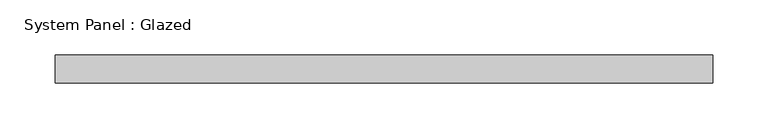
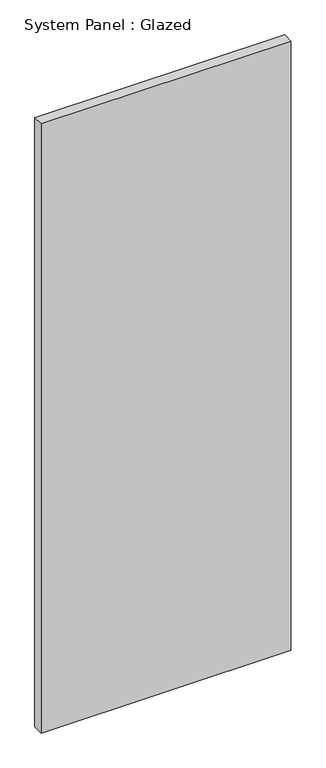
"""IFC4 building model written with IfcOpenShell, lengths in millimetres: plate geometry, System Panel : Glazed."""

from ifc_helpers import new_model, si_unit, origin, origin_with_axes, place, context, project, spatial, polyline, outline, extrude, source, transform, mapped, element, save


def system_panel_glazed_4691d008(model_context):
    return source(origin(), model_context, "Body", "SweptSolid", [
        extrude(outline(polyline([(298.45, 19.05), (-298.45, 19.05), (-298.45, 44.45), (298.45, 44.45), (298.45, 19.05)])), origin_with_axes(), (0.0, 0.0, 1.0), 1536.8745067),
    ])


if __name__ == "__main__":
    model = new_model("IFC4")
    model_context = context("Model", 3, world=origin())
    ifc_project = project(units=[si_unit("LENGTHUNIT", "METRE", prefix="MILLI")], contexts=[model_context])
    site = spatial("IfcSite", under=ifc_project)
    building = spatial("IfcBuilding", under=site)
    placement = place(None, origin())
    system_panel_glazed_shape = system_panel_glazed_4691d008(model_context)
    element("IfcPlate", 1, ObjectType="System Panel : Glazed", at=placement, inside=building, context=model_context, shape_type="MappedRepresentation", body=[
        mapped(system_panel_glazed_shape, transform((0.0, 0.0, 0.0), x_axis=(1.0, 0.0, 0.0), y_axis=(0.0, 1.0, 0.0), z_axis=(0.0, 0.0, 1.0))),
    ])
    save(model, "model.ifc")

# Revit data of these elements
# Type "System Panel : Glazed"
#   Construction Type Id = "GSP4R"
#   Analytic Construction = "1/8 in Pilkington single glazing"
#   Visual Light Transmittance = 0.9
#   Solar Heat Gain Coefficient = 0.86
#   Heat Transfer Coefficient (U) = 1.18115 BTU/(h·ft²·°F)
#   Define Thermal Properties by = 1
# Element 1 (IfcPlate, "System Panel : Glazed")
#   Materials on its faces: "Glass"
# Materials
#   "Glass": class "Glass", colour RGB 0 128 192, transparency 0.75, Description = "Soda Lime Glass", Cost = 0
